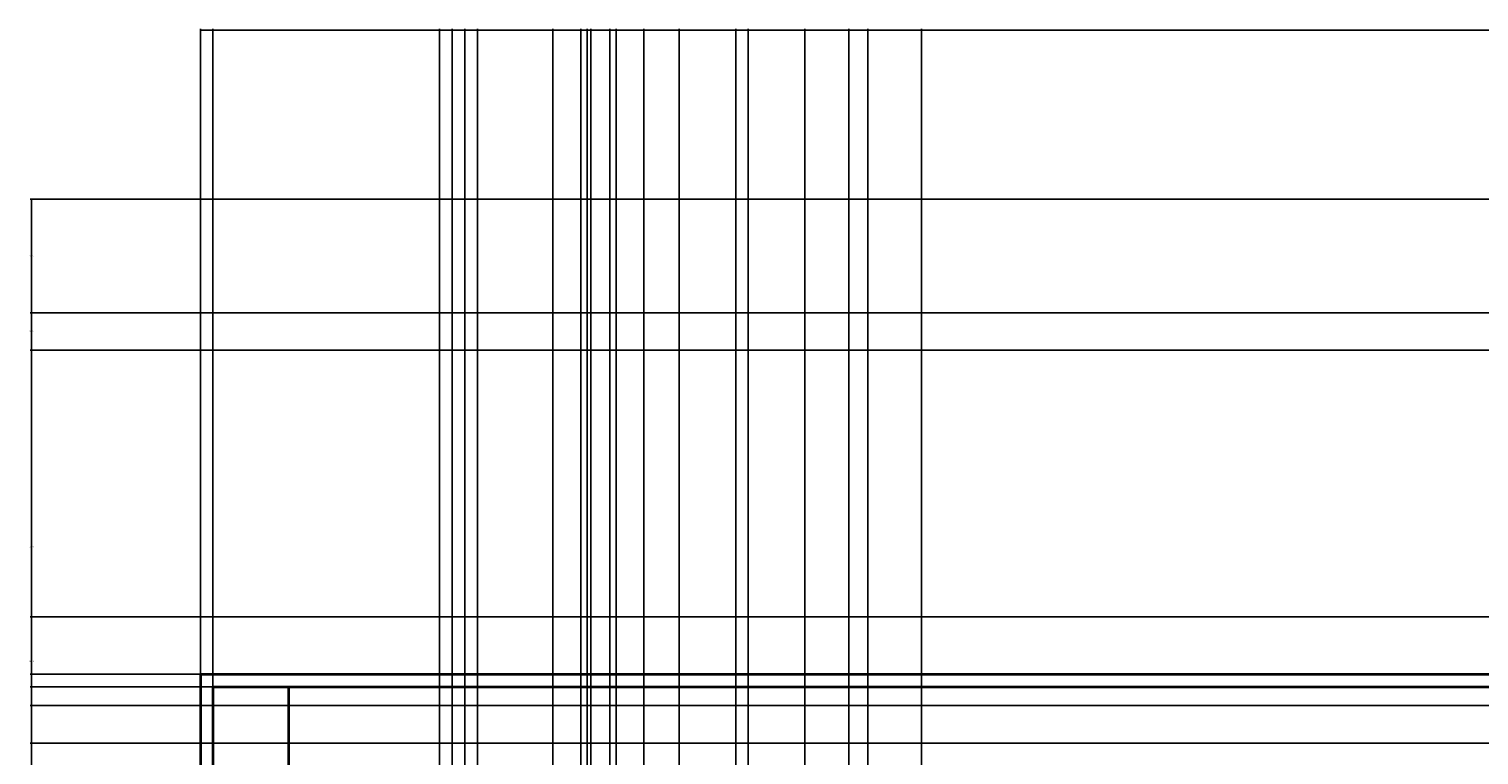
# Model space of a CAD drawing. Units: inches. Extents: x 2154 to 2740, y 571 to 1084.
# Tile 5 of 13: x 2154 to 2384, y 969 to 1084. Entities that reach past the tile are written whole.
import ezdxf

# ---------------------------------------------------------------- set-up
doc = ezdxf.new("R2010")
doc.units = ezdxf.units.IN
for name, color, linetype, lineweight in [('A-ANNO-DIMS', 2, 'Continuous', 18), ('A-ELEV', 7, 'Continuous', 35), ('A-ROOF', 1, 'Continuous', 35)]:
    doc.layers.add(name, color=color, linetype=linetype, lineweight=lineweight)
doc.styles.get("Standard").update_dxf_attribs({"font": 'arial.ttf'})
doc.dimstyles.get("Standard").update_dxf_attribs({"dimtxt": 0.18, "dimasz": 0.18, "dimexe": 0.18, "dimexo": 0.0625, "dimgap": 0.09, "dimtad": 0, "dimtih": 1, "dimtoh": 1, "dimdec": 4, "dimzin": 0, "dimdsep": 46, "dimtxsty": 'Standard', "dimcen": 0.09, "dimadec": 0, "dimazin": 0, "dimtfac": 1, "dimtdec": 4, "dimtofl": 0, "dimtmove": 0, "dimatfit": 3, "dimfxl": 1, "dimtolj": 1, "dimtzin": 0, "dimarcsym": 0})

# ---------------------------------------------------------------- blocks, each defined once
blk = doc.blocks.new('*D7')
at = {"layer": 'A-ANNO-DIMS', "color": 0, "lineweight": -2, "transparency": 16777216}
for p, q in [((2181.21, 981.59), (2181.21, 1084.04)), ((2181.39, 1083.86), (2446.92, 1083.86)), ((2713.03, 1083.86), (2447.49, 1083.86)), ((2713.21, 981.59), (2713.21, 1084.04))]:
    blk.add_line(p, q, dxfattribs=at)
at = {"layer": 'A-ANNO-DIMS', "color": 0, "transparency": 16777216}
for points in [[(2181.39, 1083.89), (2181.39, 1083.83), (2181.21, 1083.86)], [(2713.03, 1083.89), (2713.03, 1083.83), (2713.21, 1083.86)]]:
    blk.add_solid(points, dxfattribs=at)
at = {"layer": 'Defpoints', "color": 0, "transparency": 16777216}
for p in [(2713.21, 1083.86), (2181.21, 981.53), (2713.21, 981.53)]:
    blk.add_point(p, dxfattribs=at)
at = {"layer": 'A-ANNO-DIMS', "color": 0, "transparency": 16777216, "insert": (2447.21, 1083.86), "char_height": 0.18, "attachment_point": 5}
blk.add_mtext('\\A1;532', dxfattribs=at)
blk = doc.blocks.new('*D10')
at = {"layer": 'A-ANNO-DIMS', "color": 0, "lineweight": -2, "transparency": 16777216}
for p, q in [((2447.14, 1057.01), (2154.18, 1057.01)), ((2154.36, 1056.83), (2154.36, 827.45)), ((2154.36, 597.71), (2154.36, 827.09)), ((2181.14, 597.53), (2154.18, 597.53))]:
    blk.add_line(p, q, dxfattribs=at)
at = {"layer": 'A-ANNO-DIMS', "color": 0, "transparency": 16777216}
for points in [[(2154.33, 1056.83), (2154.39, 1056.83), (2154.36, 1057.01)], [(2154.33, 597.71), (2154.39, 597.71), (2154.36, 597.53)]]:
    blk.add_solid(points, dxfattribs=at)
at = {"layer": 'Defpoints', "color": 0, "transparency": 16777216}
for p in [(2154.36, 1057.01), (2447.21, 1057.01), (2181.21, 597.53)]:
    blk.add_point(p, dxfattribs=at)
at = {"layer": 'A-ANNO-DIMS', "color": 0, "transparency": 16777216, "insert": (2154.36, 827.27), "char_height": 0.18, "attachment_point": 5}
blk.add_mtext('\\A1;459.5', dxfattribs=at)
blk = doc.blocks.new('*D34')
at = {"layer": 'A-ANNO-DIMS', "color": 0, "lineweight": -2, "transparency": 16777216}
for p, q in [((2417.14, 1033.01), (2154.18, 1033.01)), ((2154.36, 1032.83), (2154.36, 1001.96)), ((2154.36, 970.71), (2154.36, 1001.59)), ((2417.14, 970.53), (2154.18, 970.53))]:
    blk.add_line(p, q, dxfattribs=at)
at = {"layer": 'A-ANNO-DIMS', "color": 0, "transparency": 16777216}
for points in [[(2154.33, 1032.83), (2154.39, 1032.83), (2154.36, 1033.01)], [(2154.33, 970.71), (2154.39, 970.71), (2154.36, 970.53)]]:
    blk.add_solid(points, dxfattribs=at)
at = {"layer": 'Defpoints', "color": 0, "transparency": 16777216}
for p in [(2154.36, 1033.01), (2417.21, 1033.01), (2417.21, 970.53)]:
    blk.add_point(p, dxfattribs=at)
at = {"layer": 'A-ANNO-DIMS', "color": 0, "transparency": 16777216, "insert": (2154.36, 1001.77), "char_height": 0.18, "attachment_point": 5}
blk.add_mtext('\\A1;62.48', dxfattribs=at)
blk = doc.blocks.new('*D39')
at = {"layer": 'A-ANNO-DIMS', "color": 0, "lineweight": -2, "transparency": 16777216}
for p, q in [((2183.21, 979.47), (2183.21, 570.5)), ((2417.21, 970.47), (2417.21, 570.5)), ((2183.39, 570.68), (2299.92, 570.68)), ((2417.03, 570.68), (2300.5, 570.68))]:
    blk.add_line(p, q, dxfattribs=at)
at = {"layer": 'A-ANNO-DIMS', "color": 0, "transparency": 16777216}
for points in [[(2183.39, 570.71), (2183.39, 570.65), (2183.21, 570.68)], [(2417.03, 570.71), (2417.03, 570.65), (2417.21, 570.68)]]:
    blk.add_solid(points, dxfattribs=at)
at = {"layer": 'Defpoints', "color": 0, "transparency": 16777216}
for p in [(2183.21, 979.53), (2417.21, 970.53), (2417.21, 570.68)]:
    blk.add_point(p, dxfattribs=at)
at = {"layer": 'A-ANNO-DIMS', "color": 0, "transparency": 16777216, "insert": (2300.21, 570.68), "char_height": 0.18, "attachment_point": 5}
blk.add_mtext('\\A1;234', dxfattribs=at)
blk = doc.blocks.new('*D48')
at = {"layer": 'A-ANNO-DIMS', "color": 0, "lineweight": -2, "transparency": 16777216}
for p, q in [((2195.27, 979.53), (2740.24, 979.53)), ((2740.06, 979.35), (2740.06, 949.71)), ((2740.06, 919.71), (2740.06, 949.35)), ((2195.27, 919.53), (2740.24, 919.53))]:
    blk.add_line(p, q, dxfattribs=at)
at = {"layer": 'A-ANNO-DIMS', "color": 0, "transparency": 16777216}
for points in [[(2740.03, 979.35), (2740.09, 979.35), (2740.06, 979.53)], [(2740.03, 919.71), (2740.09, 919.71), (2740.06, 919.53)]]:
    blk.add_solid(points, dxfattribs=at)
at = {"layer": 'Defpoints', "color": 0, "transparency": 16777216}
for p in [(2195.21, 979.53), (2740.06, 979.53), (2195.21, 919.53)]:
    blk.add_point(p, dxfattribs=at)
at = {"layer": 'A-ANNO-DIMS', "color": 0, "transparency": 16777216, "insert": (2740.06, 949.53), "char_height": 0.18, "attachment_point": 5}
blk.add_mtext('\\A1;60', dxfattribs=at)
blk = doc.blocks.new('*D49')
at = {"layer": 'A-ANNO-DIMS', "color": 0, "lineweight": -2, "transparency": 16777216}
for p, q in [((2181.14, 981.53), (2154.18, 981.53)), ((2154.36, 981.35), (2154.36, 980.71)), ((2183.14, 979.53), (2154.18, 979.53)), ((2154.36, 979.71), (2154.36, 980.35))]:
    blk.add_line(p, q, dxfattribs=at)
at = {"layer": 'A-ANNO-DIMS', "color": 0, "transparency": 16777216}
for points in [[(2154.33, 981.35), (2154.39, 981.35), (2154.36, 981.53)], [(2154.33, 979.71), (2154.39, 979.71), (2154.36, 979.53)]]:
    blk.add_solid(points, dxfattribs=at)
at = {"layer": 'Defpoints', "color": 0, "transparency": 16777216}
for p in [(2181.21, 981.53), (2154.36, 979.53), (2183.21, 979.53)]:
    blk.add_point(p, dxfattribs=at)
at = {"layer": 'A-ANNO-DIMS', "color": 0, "transparency": 16777216, "insert": (2154.36, 980.53), "char_height": 0.18, "attachment_point": 5}
blk.add_mtext('\\A1;2', dxfattribs=at)
blk = doc.blocks.new('*D50')
at = {"layer": 'A-ANNO-DIMS', "color": 0, "lineweight": -2, "transparency": 16777216}
for p, q in [((2181.21, 981.59), (2181.21, 1084.04)), ((2181.39, 1083.86), (2182.06, 1083.86)), ((2183.03, 1083.86), (2182.36, 1083.86)), ((2183.21, 979.59), (2183.21, 1084.04))]:
    blk.add_line(p, q, dxfattribs=at)
at = {"layer": 'A-ANNO-DIMS', "color": 0, "transparency": 16777216}
for points in [[(2181.39, 1083.89), (2181.39, 1083.83), (2181.21, 1083.86)], [(2183.03, 1083.89), (2183.03, 1083.83), (2183.21, 1083.86)]]:
    blk.add_solid(points, dxfattribs=at)
at = {"layer": 'Defpoints', "color": 0, "transparency": 16777216}
for p in [(2183.21, 1083.86), (2181.21, 981.53), (2183.21, 979.53)]:
    blk.add_point(p, dxfattribs=at)
at = {"layer": 'A-ANNO-DIMS', "color": 0, "transparency": 16777216, "insert": (2182.21, 1083.86), "char_height": 0.18, "attachment_point": 5}
blk.add_mtext('\\A1;2', dxfattribs=at)
blk = doc.blocks.new('*D51')
at = {"layer": 'A-ANNO-DIMS', "color": 0, "lineweight": -2, "transparency": 16777216}
for p, q in [((2183.21, 979.47), (2183.21, 570.5)), ((2195.21, 979.47), (2195.21, 570.5)), ((2183.39, 570.68), (2189, 570.68)), ((2195.03, 570.68), (2189.42, 570.68))]:
    blk.add_line(p, q, dxfattribs=at)
at = {"layer": 'A-ANNO-DIMS', "color": 0, "transparency": 16777216}
for points in [[(2183.39, 570.71), (2183.39, 570.65), (2183.21, 570.68)], [(2195.03, 570.71), (2195.03, 570.65), (2195.21, 570.68)]]:
    blk.add_solid(points, dxfattribs=at)
at = {"layer": 'Defpoints', "color": 0, "transparency": 16777216}
for p in [(2183.21, 979.53), (2195.21, 979.53), (2195.21, 570.68)]:
    blk.add_point(p, dxfattribs=at)
at = {"layer": 'A-ANNO-DIMS', "color": 0, "transparency": 16777216, "insert": (2189.21, 570.68), "char_height": 0.18, "attachment_point": 5}
blk.add_mtext('\\A1;12', dxfattribs=at)
blk = doc.blocks.new('*D53')
at = {"layer": 'A-ANNO-DIMS', "color": 0, "lineweight": -2, "transparency": 16777216}
for p, q in [((2284.21, 926.63), (2284.21, 1084.04)), ((2284.39, 1083.86), (2289.53, 1083.86)), ((2295.59, 1083.86), (2290.45, 1083.86)), ((2295.77, 920.21), (2295.77, 1084.04))]:
    blk.add_line(p, q, dxfattribs=at)
at = {"layer": 'A-ANNO-DIMS', "color": 0, "transparency": 16777216}
for points in [[(2284.39, 1083.89), (2284.39, 1083.83), (2284.21, 1083.86)], [(2295.59, 1083.89), (2295.59, 1083.83), (2295.77, 1083.86)]]:
    blk.add_solid(points, dxfattribs=at)
at = {"layer": 'Defpoints', "color": 0, "transparency": 16777216}
for p in [(2295.77, 1083.86), (2284.21, 926.56), (2295.77, 920.15)]:
    blk.add_point(p, dxfattribs=at)
at = {"layer": 'A-ANNO-DIMS', "color": 0, "transparency": 16777216, "insert": (2289.99, 1083.86), "char_height": 0.18, "attachment_point": 5}
blk.add_mtext('\\A1;11.566', dxfattribs=at)
blk = doc.blocks.new('*D62')
at = {"layer": 'A-ANNO-DIMS', "color": 0, "lineweight": -2, "transparency": 16777216}
for p, q in [((2219.21, 777.59), (2219.21, 1084.04)), ((2219.39, 1083.86), (2220.06, 1083.86)), ((2221.03, 1083.86), (2220.36, 1083.86)), ((2221.21, 777.59), (2221.21, 1084.04))]:
    blk.add_line(p, q, dxfattribs=at)
at = {"layer": 'A-ANNO-DIMS', "color": 0, "transparency": 16777216}
for points in [[(2219.39, 1083.89), (2219.39, 1083.83), (2219.21, 1083.86)], [(2221.03, 1083.89), (2221.03, 1083.83), (2221.21, 1083.86)]]:
    blk.add_solid(points, dxfattribs=at)
at = {"layer": 'Defpoints', "color": 0, "transparency": 16777216}
for p in [(2221.21, 1083.86), (2219.21, 777.53), (2221.21, 777.53)]:
    blk.add_point(p, dxfattribs=at)
at = {"layer": 'A-ANNO-DIMS', "color": 0, "transparency": 16777216, "insert": (2220.21, 1083.86), "char_height": 0.18, "attachment_point": 5}
blk.add_mtext('\\A1;2', dxfattribs=at)
blk = doc.blocks.new('*D63')
at = {"layer": 'A-ANNO-DIMS', "color": 0, "lineweight": -2, "transparency": 16777216}
for p, q in [((2221.21, 777.59), (2221.21, 1084.04)), ((2221.39, 1083.86), (2222.06, 1083.86)), ((2223.03, 1083.86), (2222.36, 1083.86)), ((2223.21, 777.59), (2223.21, 1084.04))]:
    blk.add_line(p, q, dxfattribs=at)
at = {"layer": 'A-ANNO-DIMS', "color": 0, "transparency": 16777216}
for points in [[(2221.39, 1083.89), (2221.39, 1083.83), (2221.21, 1083.86)], [(2223.03, 1083.89), (2223.03, 1083.83), (2223.21, 1083.86)]]:
    blk.add_solid(points, dxfattribs=at)
at = {"layer": 'Defpoints', "color": 0, "transparency": 16777216}
for p in [(2223.21, 1083.86), (2221.21, 777.53), (2223.21, 777.53)]:
    blk.add_point(p, dxfattribs=at)
at = {"layer": 'A-ANNO-DIMS', "color": 0, "transparency": 16777216, "insert": (2222.21, 1083.86), "char_height": 0.18, "attachment_point": 5}
blk.add_mtext('\\A1;2', dxfattribs=at)
blk = doc.blocks.new('*D64')
at = {"layer": 'A-ANNO-DIMS', "color": 0, "lineweight": -2, "transparency": 16777216}
for p, q in [((2223.21, 777.59), (2223.21, 1084.04)), ((2223.39, 1083.86), (2224.06, 1083.86)), ((2225.03, 1083.86), (2224.36, 1083.86)), ((2225.21, 777.59), (2225.21, 1084.04))]:
    blk.add_line(p, q, dxfattribs=at)
at = {"layer": 'A-ANNO-DIMS', "color": 0, "transparency": 16777216}
for points in [[(2223.39, 1083.89), (2223.39, 1083.83), (2223.21, 1083.86)], [(2225.03, 1083.89), (2225.03, 1083.83), (2225.21, 1083.86)]]:
    blk.add_solid(points, dxfattribs=at)
at = {"layer": 'Defpoints', "color": 0, "transparency": 16777216}
for p in [(2225.21, 1083.86), (2223.21, 777.53), (2225.21, 777.53)]:
    blk.add_point(p, dxfattribs=at)
at = {"layer": 'A-ANNO-DIMS', "color": 0, "transparency": 16777216, "insert": (2224.21, 1083.86), "char_height": 0.18, "attachment_point": 5}
blk.add_mtext('\\A1;2', dxfattribs=at)
blk = doc.blocks.new('*D65')
at = {"layer": 'A-ANNO-DIMS', "color": 0, "lineweight": -2, "transparency": 16777216}
for p, q in [((2225.21, 777.59), (2225.21, 1084.04)), ((2225.39, 1083.86), (2231, 1083.86)), ((2237.03, 1083.86), (2231.42, 1083.86)), ((2237.21, 777.59), (2237.21, 1084.04))]:
    blk.add_line(p, q, dxfattribs=at)
at = {"layer": 'A-ANNO-DIMS', "color": 0, "transparency": 16777216}
for points in [[(2225.39, 1083.89), (2225.39, 1083.83), (2225.21, 1083.86)], [(2237.03, 1083.89), (2237.03, 1083.83), (2237.21, 1083.86)]]:
    blk.add_solid(points, dxfattribs=at)
at = {"layer": 'Defpoints', "color": 0, "transparency": 16777216}
for p in [(2237.21, 1083.86), (2225.21, 777.53), (2237.21, 777.53)]:
    blk.add_point(p, dxfattribs=at)
at = {"layer": 'A-ANNO-DIMS', "color": 0, "transparency": 16777216, "insert": (2231.21, 1083.86), "char_height": 0.18, "attachment_point": 5}
blk.add_mtext('\\A1;12', dxfattribs=at)
blk = doc.blocks.new('*D67')
at = {"layer": 'A-ANNO-DIMS', "color": 0, "lineweight": -2, "transparency": 16777216}
for p, q in [((2411.14, 1038.96), (2154.18, 1038.96)), ((2154.36, 1038.78), (2154.36, 1036.17)), ((2154.36, 1033.19), (2154.36, 1035.8)), ((2411.14, 1033.01), (2154.18, 1033.01))]:
    blk.add_line(p, q, dxfattribs=at)
at = {"layer": 'A-ANNO-DIMS', "color": 0, "transparency": 16777216}
for points in [[(2154.33, 1038.78), (2154.39, 1038.78), (2154.36, 1038.96)], [(2154.33, 1033.19), (2154.39, 1033.19), (2154.36, 1033.01)]]:
    blk.add_solid(points, dxfattribs=at)
at = {"layer": 'Defpoints', "color": 0, "transparency": 16777216}
for p in [(2154.36, 1038.96), (2411.21, 1038.96), (2411.21, 1033.01)]:
    blk.add_point(p, dxfattribs=at)
at = {"layer": 'A-ANNO-DIMS', "color": 0, "transparency": 16777216, "insert": (2154.36, 1035.99), "char_height": 0.18, "attachment_point": 5}
blk.add_mtext('\\A1;5.941', dxfattribs=at)
blk = doc.blocks.new('*D68')
at = {"layer": 'A-ANNO-DIMS', "color": 0, "lineweight": -2, "transparency": 16777216}
for p, q in [((2447.14, 1057.01), (2154.18, 1057.01)), ((2154.36, 1056.83), (2154.36, 1048.16)), ((2154.36, 1039.14), (2154.36, 1047.8)), ((2411.14, 1038.96), (2154.18, 1038.96))]:
    blk.add_line(p, q, dxfattribs=at)
at = {"layer": 'A-ANNO-DIMS', "color": 0, "transparency": 16777216}
for points in [[(2154.33, 1056.83), (2154.39, 1056.83), (2154.36, 1057.01)], [(2154.33, 1039.14), (2154.39, 1039.14), (2154.36, 1038.96)]]:
    blk.add_solid(points, dxfattribs=at)
at = {"layer": 'Defpoints', "color": 0, "transparency": 16777216}
for p in [(2154.36, 1057.01), (2447.21, 1057.01), (2411.21, 1038.96)]:
    blk.add_point(p, dxfattribs=at)
at = {"layer": 'A-ANNO-DIMS', "color": 0, "transparency": 16777216, "insert": (2154.36, 1047.98), "char_height": 0.18, "attachment_point": 5}
blk.add_mtext('\\A1;18.05', dxfattribs=at)
blk = doc.blocks.new('*D77')
at = {"layer": 'A-ANNO-DIMS', "color": 0, "lineweight": -2, "transparency": 16777216}
for p, q in [((2434.39, 990.64), (2154.18, 990.64)), ((2154.36, 990.46), (2154.36, 983.77)), ((2154.36, 976.71), (2154.36, 983.4)), ((2420.14, 976.53), (2154.18, 976.53))]:
    blk.add_line(p, q, dxfattribs=at)
at = {"layer": 'A-ANNO-DIMS', "color": 0, "transparency": 16777216}
for points in [[(2154.33, 990.46), (2154.39, 990.46), (2154.36, 990.64)], [(2154.33, 976.71), (2154.39, 976.71), (2154.36, 976.53)]]:
    blk.add_solid(points, dxfattribs=at)
at = {"layer": 'Defpoints', "color": 0, "transparency": 16777216}
for p in [(2154.36, 990.64), (2434.46, 990.64), (2420.21, 976.53)]:
    blk.add_point(p, dxfattribs=at)
at = {"layer": 'A-ANNO-DIMS', "color": 0, "transparency": 16777216, "insert": (2154.36, 983.58), "char_height": 0.18, "attachment_point": 5}
blk.add_mtext('\\A1;14.104', dxfattribs=at)
blk = doc.blocks.new('*D110')
at = {"layer": 'A-ANNO-DIMS', "color": 0, "lineweight": -2, "transparency": 16777216}
for p, q in [((2237.21, 823.59), (2237.21, 1084.04)), ((2237.39, 1083.86), (2239.91, 1083.86)), ((2243.08, 1083.86), (2240.56, 1083.86)), ((2243.26, 823.59), (2243.26, 1084.04))]:
    blk.add_line(p, q, dxfattribs=at)
at = {"layer": 'A-ANNO-DIMS', "color": 0, "transparency": 16777216}
for points in [[(2237.39, 1083.89), (2237.39, 1083.83), (2237.21, 1083.86)], [(2243.08, 1083.89), (2243.08, 1083.83), (2243.26, 1083.86)]]:
    blk.add_solid(points, dxfattribs=at)
at = {"layer": 'Defpoints', "color": 0, "transparency": 16777216}
for p in [(2243.26, 1083.86), (2237.21, 823.53), (2243.26, 823.53)]:
    blk.add_point(p, dxfattribs=at)
at = {"layer": 'A-ANNO-DIMS', "color": 0, "transparency": 16777216, "insert": (2240.23, 1083.86), "char_height": 0.18, "attachment_point": 5}
blk.add_mtext('\\A1;6.05', dxfattribs=at)
blk = doc.blocks.new('*D111')
at = {"layer": 'A-ANNO-DIMS', "color": 0, "lineweight": -2, "transparency": 16777216}
for p, q in [((2243.26, 873.59), (2243.26, 1084.04)), ((2243.44, 1083.86), (2244.61, 1083.86)), ((2246.08, 1083.86), (2244.91, 1083.86)), ((2246.26, 870.59), (2246.26, 1084.04))]:
    blk.add_line(p, q, dxfattribs=at)
at = {"layer": 'A-ANNO-DIMS', "color": 0, "transparency": 16777216}
for points in [[(2243.44, 1083.89), (2243.44, 1083.83), (2243.26, 1083.86)], [(2246.08, 1083.89), (2246.08, 1083.83), (2246.26, 1083.86)]]:
    blk.add_solid(points, dxfattribs=at)
at = {"layer": 'Defpoints', "color": 0, "transparency": 16777216}
for p in [(2246.26, 1083.86), (2243.26, 873.53), (2246.26, 870.53)]:
    blk.add_point(p, dxfattribs=at)
at = {"layer": 'A-ANNO-DIMS', "color": 0, "transparency": 16777216, "insert": (2244.76, 1083.86), "char_height": 0.18, "attachment_point": 5}
blk.add_mtext('\\A1;3', dxfattribs=at)
blk = doc.blocks.new('*D113')
at = {"layer": 'A-ANNO-DIMS', "color": 0, "lineweight": -2, "transparency": 16777216}
for p, q in [((2246.26, 870.59), (2246.26, 1084.04)), ((2246.44, 1083.86), (2246.63, 1083.86)), ((2247.08, 1083.86), (2246.88, 1083.86)), ((2247.26, 869.59), (2247.26, 1084.04))]:
    blk.add_line(p, q, dxfattribs=at)
at = {"layer": 'A-ANNO-DIMS', "color": 0, "transparency": 16777216}
for points in [[(2246.44, 1083.89), (2246.44, 1083.83), (2246.26, 1083.86)], [(2247.08, 1083.89), (2247.08, 1083.83), (2247.26, 1083.86)]]:
    blk.add_solid(points, dxfattribs=at)
at = {"layer": 'Defpoints', "color": 0, "transparency": 16777216}
for p in [(2247.26, 1083.86), (2246.26, 870.53), (2247.26, 869.53)]:
    blk.add_point(p, dxfattribs=at)
at = {"layer": 'A-ANNO-DIMS', "color": 0, "transparency": 16777216, "insert": (2246.76, 1083.86), "char_height": 0.18, "attachment_point": 5}
blk.add_mtext('\\A1;1', dxfattribs=at)
blk = doc.blocks.new('*D114')
at = {"layer": 'A-ANNO-DIMS', "color": 0, "lineweight": -2, "transparency": 16777216}
for p, q in [((2247.26, 869.59), (2247.26, 1084.04)), ((2247.44, 1083.86), (2252.05, 1083.86)), ((2257.08, 1083.86), (2252.47, 1083.86)), ((2257.26, 869.59), (2257.26, 1084.04))]:
    blk.add_line(p, q, dxfattribs=at)
at = {"layer": 'A-ANNO-DIMS', "color": 0, "transparency": 16777216}
for points in [[(2247.44, 1083.89), (2247.44, 1083.83), (2247.26, 1083.86)], [(2257.08, 1083.89), (2257.08, 1083.83), (2257.26, 1083.86)]]:
    blk.add_solid(points, dxfattribs=at)
at = {"layer": 'Defpoints', "color": 0, "transparency": 16777216}
for p in [(2257.26, 1083.86), (2247.26, 869.53), (2257.26, 869.53)]:
    blk.add_point(p, dxfattribs=at)
at = {"layer": 'A-ANNO-DIMS', "color": 0, "transparency": 16777216, "insert": (2252.26, 1083.86), "char_height": 0.18, "attachment_point": 5}
blk.add_mtext('\\A1;10', dxfattribs=at)
blk = doc.blocks.new('*D115')
at = {"layer": 'A-ANNO-DIMS', "color": 0, "lineweight": -2, "transparency": 16777216}
for p, q in [((2257.26, 869.59), (2257.26, 1084.04)), ((2257.44, 1083.86), (2261.61, 1083.86)), ((2266.08, 1083.86), (2261.91, 1083.86)), ((2266.26, 869.59), (2266.26, 1084.04))]:
    blk.add_line(p, q, dxfattribs=at)
at = {"layer": 'A-ANNO-DIMS', "color": 0, "transparency": 16777216}
for points in [[(2257.44, 1083.89), (2257.44, 1083.83), (2257.26, 1083.86)], [(2266.08, 1083.89), (2266.08, 1083.83), (2266.26, 1083.86)]]:
    blk.add_solid(points, dxfattribs=at)
at = {"layer": 'Defpoints', "color": 0, "transparency": 16777216}
for p in [(2266.26, 1083.86), (2257.26, 869.53), (2266.26, 869.53)]:
    blk.add_point(p, dxfattribs=at)
at = {"layer": 'A-ANNO-DIMS', "color": 0, "transparency": 16777216, "insert": (2261.76, 1083.86), "char_height": 0.18, "attachment_point": 5}
blk.add_mtext('\\A1;9', dxfattribs=at)
blk = doc.blocks.new('*D116')
at = {"layer": 'A-ANNO-DIMS', "color": 0, "lineweight": -2, "transparency": 16777216}
for p, q in [((2266.26, 869.59), (2266.26, 1084.04)), ((2266.44, 1083.86), (2267.11, 1083.86)), ((2268.08, 1083.86), (2267.41, 1083.86)), ((2268.26, 869.59), (2268.26, 1084.04))]:
    blk.add_line(p, q, dxfattribs=at)
at = {"layer": 'A-ANNO-DIMS', "color": 0, "transparency": 16777216}
for points in [[(2266.44, 1083.89), (2266.44, 1083.83), (2266.26, 1083.86)], [(2268.08, 1083.89), (2268.08, 1083.83), (2268.26, 1083.86)]]:
    blk.add_solid(points, dxfattribs=at)
at = {"layer": 'Defpoints', "color": 0, "transparency": 16777216}
for p in [(2268.26, 1083.86), (2266.26, 869.53), (2268.26, 869.53)]:
    blk.add_point(p, dxfattribs=at)
at = {"layer": 'A-ANNO-DIMS', "color": 0, "transparency": 16777216, "insert": (2267.26, 1083.86), "char_height": 0.18, "attachment_point": 5}
blk.add_mtext('\\A1;2', dxfattribs=at)
blk = doc.blocks.new('*D117')
at = {"layer": 'A-ANNO-DIMS', "color": 0, "lineweight": -2, "transparency": 16777216}
for p, q in [((2268.26, 869.59), (2268.26, 1084.04)), ((2268.44, 1083.86), (2272.61, 1083.86)), ((2277.08, 1083.86), (2272.91, 1083.86)), ((2277.26, 869.59), (2277.26, 1084.04))]:
    blk.add_line(p, q, dxfattribs=at)
at = {"layer": 'A-ANNO-DIMS', "color": 0, "transparency": 16777216}
for points in [[(2268.44, 1083.89), (2268.44, 1083.83), (2268.26, 1083.86)], [(2277.08, 1083.89), (2277.08, 1083.83), (2277.26, 1083.86)]]:
    blk.add_solid(points, dxfattribs=at)
at = {"layer": 'Defpoints', "color": 0, "transparency": 16777216}
for p in [(2277.26, 1083.86), (2268.26, 869.53), (2277.26, 869.53)]:
    blk.add_point(p, dxfattribs=at)
at = {"layer": 'A-ANNO-DIMS', "color": 0, "transparency": 16777216, "insert": (2272.76, 1083.86), "char_height": 0.18, "attachment_point": 5}
blk.add_mtext('\\A1;9', dxfattribs=at)
blk = doc.blocks.new('*D118')
at = {"layer": 'A-ANNO-DIMS', "color": 0, "lineweight": -2, "transparency": 16777216}
for p, q in [((2277.26, 869.59), (2277.26, 1084.04)), ((2277.44, 1083.86), (2282.05, 1083.86)), ((2287.08, 1083.86), (2282.47, 1083.86)), ((2287.26, 869.59), (2287.26, 1084.04))]:
    blk.add_line(p, q, dxfattribs=at)
at = {"layer": 'A-ANNO-DIMS', "color": 0, "transparency": 16777216}
for points in [[(2277.44, 1083.89), (2277.44, 1083.83), (2277.26, 1083.86)], [(2287.08, 1083.89), (2287.08, 1083.83), (2287.26, 1083.86)]]:
    blk.add_solid(points, dxfattribs=at)
at = {"layer": 'Defpoints', "color": 0, "transparency": 16777216}
for p in [(2287.26, 1083.86), (2277.26, 869.53), (2287.26, 869.53)]:
    blk.add_point(p, dxfattribs=at)
at = {"layer": 'A-ANNO-DIMS', "color": 0, "transparency": 16777216, "insert": (2282.26, 1083.86), "char_height": 0.18, "attachment_point": 5}
blk.add_mtext('\\A1;10', dxfattribs=at)
blk = doc.blocks.new('*D136')
at = {"layer": 'A-ANNO-DIMS', "color": 0, "lineweight": -2, "transparency": 16777216}
for p, q in [((2241.65, 648.59), (2241.65, 1084.04)), ((2241.83, 1083.86), (2242.03, 1083.86)), ((2242.47, 1083.86), (2242.28, 1083.86)), ((2242.65, 648.59), (2242.65, 1084.04))]:
    blk.add_line(p, q, dxfattribs=at)
at = {"layer": 'A-ANNO-DIMS', "color": 0, "transparency": 16777216}
for points in [[(2241.83, 1083.89), (2241.83, 1083.83), (2241.65, 1083.86)], [(2242.47, 1083.89), (2242.47, 1083.83), (2242.65, 1083.86)]]:
    blk.add_solid(points, dxfattribs=at)
at = {"layer": 'Defpoints', "color": 0, "transparency": 16777216}
for p in [(2242.65, 1083.86), (2241.65, 648.53), (2242.65, 648.53)]:
    blk.add_point(p, dxfattribs=at)
at = {"layer": 'A-ANNO-DIMS', "color": 0, "transparency": 16777216, "insert": (2242.15, 1083.86), "char_height": 0.18, "attachment_point": 5}
blk.add_mtext('\\A1;1', dxfattribs=at)
blk = doc.blocks.new('*D137')
at = {"layer": 'A-ANNO-DIMS', "color": 0, "lineweight": -2, "transparency": 16777216}
for p, q in [((2242.65, 648.59), (2242.65, 1084.04)), ((2242.83, 1083.86), (2247, 1083.86)), ((2251.47, 1083.86), (2247.3, 1083.86)), ((2251.65, 648.59), (2251.65, 1084.04))]:
    blk.add_line(p, q, dxfattribs=at)
at = {"layer": 'A-ANNO-DIMS', "color": 0, "transparency": 16777216}
for points in [[(2242.83, 1083.89), (2242.83, 1083.83), (2242.65, 1083.86)], [(2251.47, 1083.89), (2251.47, 1083.83), (2251.65, 1083.86)]]:
    blk.add_solid(points, dxfattribs=at)
at = {"layer": 'Defpoints', "color": 0, "transparency": 16777216}
for p in [(2251.65, 1083.86), (2242.65, 648.53), (2251.65, 648.53)]:
    blk.add_point(p, dxfattribs=at)
at = {"layer": 'A-ANNO-DIMS', "color": 0, "transparency": 16777216, "insert": (2247.15, 1083.86), "char_height": 0.18, "attachment_point": 5}
blk.add_mtext('\\A1;9', dxfattribs=at)

msp = doc.modelspace()

# ---------------------------------------------------------------- linework, layer by layer
at = {"layer": 'A-ELEV'}
for p, q in [((2181.2067, 981.5321), (2181.2067, 753.5321)), ((2183.2067, 979.5321), (2183.2067, 757.5321))]:
    msp.add_line(p, q, dxfattribs=at)
at = {"layer": 'A-ROOF'}
for p, q in [((2181.2067, 981.5321), (2417.2067, 981.5321)), ((2183.2067, 979.5321), (2417.2067, 979.5321)), ((2195.2067, 979.5321), (2195.2067, 903.5321))]:
    msp.add_line(p, q, dxfattribs=at)

# ---------------------------------------------------------------- dimensions: what is measured, and where the dimension line sits
at = {"layer": 'A-ANNO-DIMS'}
for base, p1, p2, override, picture, middle in [((2713.2067, 1083.8553), (2181.2067, 981.5321), (2713.2067, 981.5321), {"dimdec": 0, "dimlfac": 1, "dimrnd": 0, "dimzin": 0, "dimdsep": 46, "dimlunit": 2}, '*D7', (2447.2067, 1083.8553)), ((2183.2067, 1083.8553), (2181.2067, 981.5321), (2183.2067, 979.5321), {"dimdec": 0, "dimlfac": 1, "dimrnd": 0, "dimzin": 0, "dimdsep": 46, "dimlunit": 2}, '*D50', (2182.2067, 1083.8553)), ((2221.2067, 1083.8553), (2219.2067, 777.5321), (2221.2067, 777.5321), {"dimdec": 0, "dimlfac": 1, "dimrnd": 0, "dimzin": 0, "dimdsep": 46, "dimlunit": 2}, '*D62', (2220.2067, 1083.8553)), ((2223.2067, 1083.8553), (2221.2067, 777.5321), (2223.2067, 777.5321), {"dimdec": 0, "dimlfac": 1, "dimrnd": 0, "dimzin": 0, "dimdsep": 46, "dimlunit": 2}, '*D63', (2222.2067, 1083.8553)), ((2225.2067, 1083.8553), (2223.2067, 777.5321), (2225.2067, 777.5321), {"dimdec": 0, "dimlfac": 1, "dimrnd": 0, "dimzin": 0, "dimdsep": 46, "dimlunit": 2}, '*D64', (2224.2067, 1083.8553)), ((2237.2067, 1083.8553), (2225.2067, 777.5321), (2237.2067, 777.5321), {"dimdec": 0, "dimlfac": 1, "dimrnd": 0, "dimzin": 0, "dimdsep": 46, "dimlunit": 2}, '*D65', (2231.2067, 1083.8553)), ((2243.2568, 1083.8553), (2237.2067, 823.5321), (2243.2568, 823.5321), {"dimdec": 2, "dimlfac": 1, "dimrnd": 0, "dimzin": 0, "dimdsep": 46, "dimlunit": 2}, '*D110', (2240.2317, 1083.8553)), ((2242.6527, 1083.8553), (2241.6527, 648.5321), (2242.6527, 648.5321), {"dimdec": 0, "dimlfac": 1, "dimrnd": 0, "dimzin": 0, "dimdsep": 46, "dimlunit": 2}, '*D136', (2242.1527, 1083.8553)), ((2251.6527, 1083.8553), (2242.6527, 648.5321), (2251.6527, 648.5321), {"dimdec": 0, "dimlfac": 1, "dimrnd": 0, "dimzin": 0, "dimdsep": 46, "dimlunit": 2}, '*D137', (2247.1527, 1083.8553)), ((2246.2568, 1083.8553), (2243.2568, 873.5321), (2246.2568, 870.5321), {"dimdec": 0, "dimlfac": 1, "dimrnd": 0, "dimzin": 0, "dimdsep": 46, "dimlunit": 2}, '*D111', (2244.7568, 1083.8553)), ((2247.2568, 1083.8553), (2246.2568, 870.5321), (2247.2568, 869.5321), {"dimdec": 0, "dimlfac": 1, "dimrnd": 0, "dimzin": 0, "dimdsep": 46, "dimlunit": 2}, '*D113', (2246.7568, 1083.8553)), ((2257.2568, 1083.8553), (2247.2568, 869.5321), (2257.2568, 869.5321), {"dimdec": 0, "dimlfac": 1, "dimrnd": 0, "dimzin": 0, "dimdsep": 46, "dimlunit": 2}, '*D114', (2252.2568, 1083.8553)), ((2266.2568, 1083.8553), (2257.2568, 869.5321), (2266.2568, 869.5321), {"dimdec": 0, "dimlfac": 1, "dimrnd": 0, "dimzin": 0, "dimdsep": 46, "dimlunit": 2}, '*D115', (2261.7568, 1083.8553)), ((2268.2568, 1083.8553), (2266.2568, 869.5321), (2268.2568, 869.5321), {"dimdec": 0, "dimlfac": 1, "dimrnd": 0, "dimzin": 0, "dimdsep": 46, "dimlunit": 2}, '*D116', (2267.2568, 1083.8553)), ((2277.2568, 1083.8553), (2268.2568, 869.5321), (2277.2568, 869.5321), {"dimdec": 0, "dimlfac": 1, "dimrnd": 0, "dimzin": 0, "dimdsep": 46, "dimlunit": 2}, '*D117', (2272.7568, 1083.8553)), ((2287.2568, 1083.8553), (2277.2568, 869.5321), (2287.2568, 869.5321), {"dimdec": 0, "dimlfac": 1, "dimrnd": 0, "dimzin": 0, "dimdsep": 46, "dimlunit": 2}, '*D118', (2282.2568, 1083.8553)), ((2295.7731, 1083.8553), (2284.2067, 926.5633), (2295.7731, 920.1485), {"dimdec": 3, "dimlfac": 1, "dimrnd": 0, "dimzin": 0, "dimdsep": 46, "dimlunit": 2}, '*D53', (2289.9899, 1083.8553)), ((2417.2067, 570.6821), (2183.2067, 979.5321), (2417.2067, 970.5321), {"dimdec": 0, "dimlfac": 1, "dimrnd": 0, "dimzin": 0, "dimdsep": 46, "dimlunit": 2}, '*D39', (2300.2067, 570.6821)), ((2195.2067, 570.6821), (2183.2067, 979.5321), (2195.2067, 979.5321), {"dimdec": 0, "dimlfac": 1, "dimrnd": 0, "dimzin": 0, "dimdsep": 46, "dimlunit": 2}, '*D51', (2189.2067, 570.6821))]:
    dim = msp.add_linear_dim(base=base, p1=p1, p2=p2, dimstyle='Standard', override=override, dxfattribs=at)
    dim.commit()
    dim.dimension.update_dxf_attribs({"geometry": picture, "text_midpoint": middle})
for base, p1, p2, override, picture, middle in [((2154.3567, 1057.0053), (2181.2067, 597.5321), (2447.2067, 1057.0053), {"dimdec": 1, "dimlfac": 1, "dimrnd": 0, "dimzin": 0, "dimdsep": 46, "dimlunit": 2}, '*D10', (2154.3567, 827.2687)), ((2154.3567, 1057.0053), (2411.2067, 1038.9557), (2447.2067, 1057.0053), {"dimdec": 2, "dimlfac": 1, "dimrnd": 0, "dimzin": 0, "dimdsep": 46, "dimlunit": 2}, '*D68', (2154.3567, 1047.9805)), ((2154.3567, 1038.9557), (2411.2067, 1033.0148), (2411.2067, 1038.9557), {"dimdec": 3, "dimlfac": 1, "dimrnd": 0, "dimzin": 0, "dimdsep": 46, "dimlunit": 2}, '*D67', (2154.3567, 1035.9852)), ((2154.3567, 1033.0148), (2417.2067, 970.5321), (2417.2067, 1033.0148), {"dimdec": 2, "dimlfac": 1, "dimrnd": 0, "dimzin": 0, "dimdsep": 46, "dimlunit": 2}, '*D34', (2154.3567, 1001.7734)), ((2154.3567, 990.6361), (2420.2067, 976.5321), (2434.4565, 990.6361), {"dimdec": 3, "dimlfac": 1, "dimrnd": 0, "dimzin": 0, "dimdsep": 46, "dimlunit": 2}, '*D77', (2154.3567, 983.5841)), ((2154.3567, 979.5321), (2181.2067, 981.5321), (2183.2067, 979.5321), {"dimdec": 0, "dimlfac": 1, "dimrnd": 0, "dimzin": 0, "dimdsep": 46, "dimlunit": 2}, '*D49', (2154.3567, 980.5321)), ((2740.0567, 979.5321), (2195.2067, 919.5321), (2195.2067, 979.5321), {"dimdec": 0, "dimlfac": 1, "dimrnd": 0, "dimzin": 0, "dimdsep": 46, "dimlunit": 2}, '*D48', (2740.0567, 949.5321))]:
    dim = msp.add_linear_dim(base=base, p1=p1, p2=p2, angle=90, dimstyle='Standard', override=override, dxfattribs=at)
    dim.commit()
    dim.dimension.update_dxf_attribs({"geometry": picture, "text_midpoint": middle})

doc.saveas('drawing.dxf')
